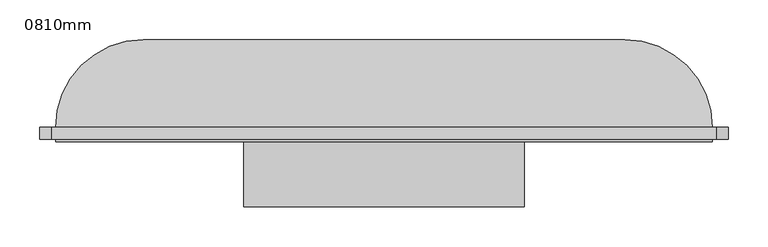
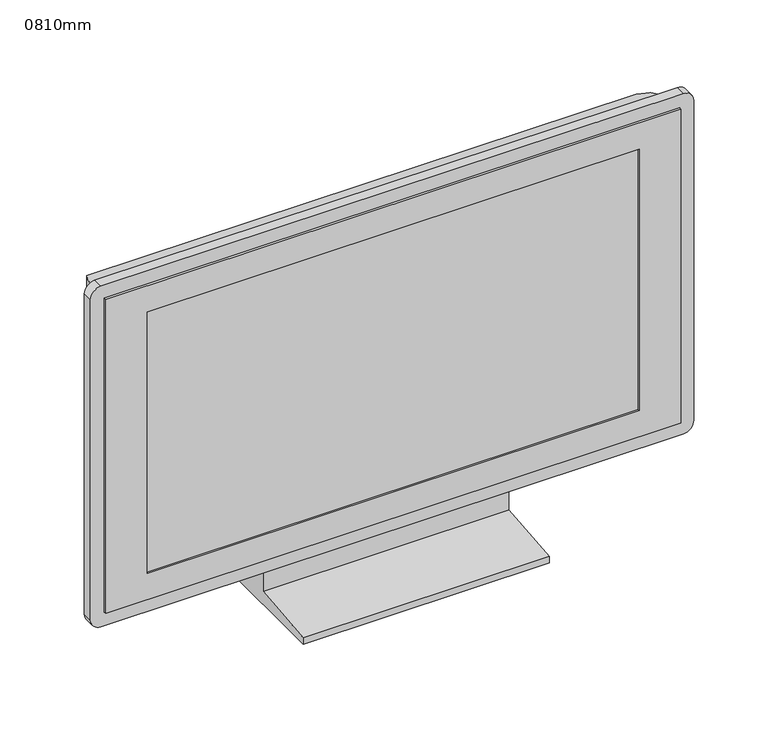
"""IFC4 building model written with IfcOpenShell, lengths in millimetres: furniture geometry, 0810mm."""

from ifc_helpers import new_model, si_unit, point, frame, frame_2d, origin, place, context, project, spatial, polyline, circle_curve, ellipse_curve, trimmed, segment, composite_curve, outline, extrude, faceted_brep, source, transform, mapped, element, save
from ifc_brep_helpers import plane_surface, cylinder_surface, advanced_brep


def furniture_0810mm_56245f3a(model_context):
    return source(origin(), model_context, "Body", "SolidModel", [
        extrude(outline(polyline([(-51.4613764, 80.0), (-1.4613764, 80.0), (48.5386236, 0.0), (-151.4613764, 0.0), (-151.4613764, 10.0), (-51.4613764, 20.0), (-51.4613764, 80.0)])), frame((-180.4346678, 0.0, 0.0), z_axis=(1.0, 0.0, 0.0), x_axis=(0.0, 1.0, 0.0)), (0.0, 0.0, 1.0), 352.9803073),
        faceted_brep([(409.0357931, -69.4613764, 557.1392838), (-416.9248214, -69.4613764, 557.1392838), (-416.9248214, -69.4613764, 80.0), (409.0357931, -69.4613764, 80.0), (-356.9248214, -69.4613764, 517.1392838), (349.0357931, -69.4613764, 517.1392838), (349.0357931, -69.4613764, 120.0), (-356.9248214, -69.4613764, 120.0), (409.0357931, -51.4613764, 557.1392838), (409.0357931, -51.4613764, 80.0), (-416.9248214, -51.4613764, 80.0), (-416.9248214, -51.4613764, 557.1392838), (-356.9248214, -66.4613764, 517.1392838), (-356.9248214, -66.4613764, 120.0), (349.0357931, -66.4613764, 120.0), (349.0357931, -66.4613764, 517.1392838)], [[[0, 1, 2, 3], [4, 5, 6, 7]], [[8, 9, 10, 11]], [[1, 0, 8, 11]], [[2, 1, 11, 10]], [[3, 2, 10, 9]], [[0, 3, 9, 8]], [[12, 13, 14, 15]], [[12, 15, 5, 4]], [[15, 14, 6, 5]], [[14, 13, 7, 6]], [[13, 12, 4, 7]]]),
        extrude(outline(composite_curve([segment(polyline([(577.1392838, 414.0357931), (577.1392838, -421.9248214)]), True, "CONTINUOUS"), segment(trimmed(circle_curve(frame_2d((562.1392838, -421.9248214)), 15.0), [point((577.1392838, -421.9248214))], [point((562.1392838, -436.9248214))], False, "CARTESIAN"), True, "CONTINUOUS"), segment(polyline([(562.1392838, -436.9248214), (75.0, -436.9248214)]), True, "CONTINUOUS"), segment(trimmed(circle_curve(frame_2d((75.0, -421.9248214)), 15.0), [point((75.0, -436.9248214))], [point((60.0, -421.9248214))], False, "CARTESIAN"), True, "CONTINUOUS"), segment(polyline([(60.0, -421.9248214), (60.0, 414.0357931)]), True, "CONTINUOUS"), segment(trimmed(circle_curve(frame_2d((75.0, 414.0357931)), 15.0), [point((60.0, 414.0357931))], [point((75.0, 429.0357931))], False, "CARTESIAN"), True, "CONTINUOUS"), segment(polyline([(75.0, 429.0357931), (562.1392838, 429.0357931)]), True, "CONTINUOUS"), segment(trimmed(circle_curve(frame_2d((562.1392838, 414.0357931)), 15.0), [point((562.1392838, 429.0357931))], [point((577.1392838, 414.0357931))], False, "CARTESIAN"), True, "CONTINUOUS")], self_intersect=False), holes=[polyline([(557.1392838, 409.0357931), (80.0, 409.0357931), (80.0, -416.9248214), (557.1392838, -416.9248214), (557.1392838, 409.0357931)])]), frame((0.0, -66.4613764, 0.0), z_axis=(0.0, 1.0, 0.0), x_axis=(0.0, 0.0, 1.0)), (0.0, 0.0, 1.0), 15.0),
        advanced_brep(
        [(-416.9248214, -51.4613764, 80.0), (409.0357931, -51.4613764, 80.0), (409.0357931, -51.4613764, 557.1392838), (-416.9248214, -51.4613764, 557.1392838), (299.0357931, 58.5386236, 80.0), (-306.9248214, 58.5386236, 80.0), (-306.9248214, 58.5386236, 447.1392838), (299.0357931, 58.5386236, 447.1392838)],
        [
            (0, 1),
            (1, 2),
            (2, 3),
            (3, 0),
            (4, 5),
            (5, 6),
            (6, 7),
            (7, 4),
            (0, 5, circle_curve(frame((-306.9248214, -51.4613764, 80.0), z_axis=(0.0, 0.0, -1.0), x_axis=(-1.0, 0.0, 0.0)), 110.0)),
            (4, 1, circle_curve(frame((299.0357931, -51.4613764, 80.0), z_axis=(0.0, 0.0, -1.0), x_axis=(1.0, 0.0, 0.0)), 110.0)),
            (7, 2, ellipse_curve(frame((299.0357931, -51.4613764, 447.1392838), z_axis=(0.7071067811865475, 0.0, -0.7071067811865475), x_axis=(0.7071067811865474, 0.0, 0.7071067811865476)), 155.5634919, 110.0)),
            (6, 3, ellipse_curve(frame((-306.9248214, -51.4613764, 447.1392838), z_axis=(0.7071067811865475, 0.0, 0.7071067811865475), x_axis=(-0.7071067811865476, 0.0, 0.7071067811865474)), 155.5634919, 110.0)),
        ],
        [
            plane_surface(frame((-416.9248214, -51.4613764, 557.1392838), z_axis=(0.0, -1.0, 0.0), x_axis=(-1.0, 0.0, 0.0))),
            plane_surface(frame((-416.9248214, 58.5386236, 557.1392838), z_axis=(0.0, 1.0, 0.0), x_axis=(1.0, 0.0, 0.0))),
            plane_surface(frame((-416.9248214, -51.4613764, 80.0), z_axis=(0.0, 0.0, -1.0), x_axis=(0.0, 1.0, 0.0))),
            cylinder_surface(frame((299.0357931, -51.4613764, 80.0), z_axis=(0.0, 0.0, 1.0), x_axis=(1.0, 0.0, 0.0)), 110.0),
            cylinder_surface(frame((409.0357931, -51.4613764, 447.1392838), z_axis=(-1.0, 0.0, 0.0), x_axis=(0.0, 0.0, 1.0)), 110.0),
            cylinder_surface(frame((-306.9248214, -51.4613764, 557.1392838), z_axis=(0.0, 0.0, -1.0), x_axis=(-1.0, 0.0, 0.0)), 110.0),
        ],
        [
            (0, [[1, 2, 3, 4]]),
            (1, [[5, 6, 7, 8]]),
            (2, [[-1, 9, -5, 10]]),
            (3, [[11, -2, -10, -8]]),
            (4, [[-11, -7, 12, -3]]),
            (5, [[-12, -6, -9, -4]]),
        ],
    ),
    ])


if __name__ == "__main__":
    model = new_model("IFC4")
    model_context = context("Model", 3, world=origin())
    ifc_project = project(units=[si_unit("LENGTHUNIT", "METRE", prefix="MILLI")], contexts=[model_context])
    site = spatial("IfcSite", under=ifc_project)
    building = spatial("IfcBuilding", under=site)
    placement = place(None, origin())
    furniture_0810mm_shape = furniture_0810mm_56245f3a(model_context)
    element("IfcFurniture", 1, ObjectType="0810mm", at=placement, inside=building, context=model_context, shape_type="MappedRepresentation", body=[
        mapped(furniture_0810mm_shape, transform((0.0, 0.0, 0.0), x_axis=(1.0, 0.0, 0.0), y_axis=(0.0, 1.0, 0.0), z_axis=(0.0, 0.0, 1.0))),
    ])
    save(model, "model.ifc")

# Revit data of these elements
# Type "0810mm"
#   SinAng = 0.49 mm
#   L = 705.961 mm
#   H = 397.139 mm
#   Thickness = 110 mm
#   Diagonal = 810 mm
#   CosAng = 0.872 mm
#   Stand [instance default] = yes
#   Default Elevation = 0
# Element 1 (IfcFurniture, "0810mm")
#   Materials on its faces: "TV - Black", "TV - Glass", "TV - Screen"
# Materials
#   "TV - Black": colour RGB 49 49 49, transparency 0
#   "TV - Glass": colour RGB 157 157 157, transparency 0.9
#   "TV - Screen": colour RGB 0 0 0, transparency 0
